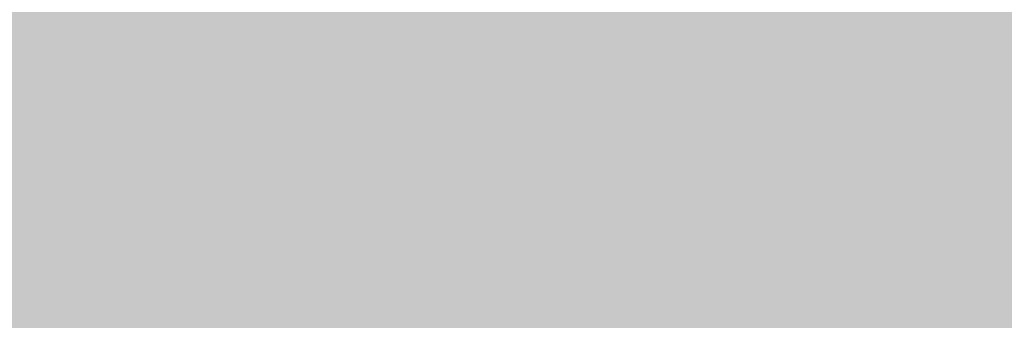
# Model space of a CAD drawing. Units: feet. Extents: x 3168 to 4724, y 827 to 1477.
# Tile 92 of 256: x 3275.224 to 3277.376, y 1098.344 to 1099.001. Entities that reach past the tile are written whole.
import ezdxf

# ---------------------------------------------------------------- set-up
doc = ezdxf.new("R2010")
doc.units = ezdxf.units.FT
doc.layers.add('A-ELEV', color=7, linetype='Continuous', lineweight=35)
doc.layers.add('A-ELEV-PATT', color=8, linetype='Continuous', lineweight=13)

msp = doc.modelspace()

# ---------------------------------------------------------------- hatches: boundary and pattern name
at = {"layer": 'A-ELEV-PATT'}
h = msp.add_hatch(color=256, dxfattribs=at)
h.dxf.hatch_style = 1
edge = h.paths.add_edge_path()
edge.add_ellipse((3552.9058, 979.2201), major_axis=(36.7449, 0), ratio=0.4848485, start_angle=0, end_angle=360)
edge = h.paths.add_edge_path()
edge.add_ellipse((3559.8916, 929.2523), major_axis=(36.7449, 0), ratio=0.4848485, start_angle=0, end_angle=360)
edge = h.paths.add_edge_path()
edge.add_line((3299.3168, 1198.6061), (3479.9167, 1198.6061))
edge.add_line((3479.9167, 1198.6061), (3479.9167, 1209.8686))
edge.add_spline(control_points=[(3479.9167, 1209.8686), (3464.3012, 1209.8686), (3448.6856, 1209.8686), (3410.9491, 1209.8686), (3388.8282, 1209.8686), (3355.6469, 1209.8686), (3344.5864, 1209.8686), (3327.9957, 1209.8686), (3322.4655, 1209.8686), (3314.1702, 1209.8686), (3311.4051, 1209.8686), (3307.2574, 1209.8686), (3305.8748, 1209.8686), (3303.801, 1209.8686), (3303.1097, 1209.8686), (3302.0728, 1209.8686), (3301.7272, 1209.8686), (3301.2087, 1209.8686), (3301.0359, 1209.8686), (3300.7767, 1209.8686), (3300.6903, 1209.8686), (3300.5606, 1209.8686), (3300.5174, 1209.8686), (3300.4526, 1209.8686), (3300.431, 1209.8686), (3300.3986, 1209.8686), (3300.3878, 1209.8686), (3300.3662, 1209.8686), (3300.3457, 1209.8686), (3300.3455, 1209.8686), (3300.3455, 1209.8686), (3300.3433, 1209.8686), (3300.3411, 1209.8686), (3300.3379, 1209.8686), (3300.3368, 1209.8686), (3300.3339, 1209.8686), (3300.3321, 1209.8686), (3300.3255, 1209.8686), (3300.3207, 1209.8686), (3300.3109, 1209.8686), (3300.306, 1209.8686), (3300.2905, 1209.8686), (3300.28, 1209.8686), (3300.2324, 1209.8688), (3300.1953, 1209.869), (3299.9511, 1209.8706), (3299.7448, 1209.8743), (3299.4368, 1209.8833), (3299.3344, 1209.8868), (3299.1811, 1209.8929), (3299.13, 1209.8951), (3298.6522, 1209.9168), (3298.2295, 1209.9457), (3297.6016, 1210.0024), (3297.3934, 1210.0235), (3297.0827, 1210.0583), (3296.9793, 1210.0705), (3296.293, 1210.1549), (3295.7181, 1210.2434), (3294.8687, 1210.3989), (3294.5877, 1210.4545), (3294.1693, 1210.5433), (3294.0304, 1210.5739), (3291.7071, 1211.1012), (3289.6536, 1211.8134), (3285.7763, 1213.564), (3283.9514, 1214.6035), (3280.5122, 1216.9801), (3278.8972, 1218.3176), (3276.3799, 1220.8295), (3275.416, 1221.9177), (3274.0393, 1223.7077), (3273.581, 1224.3495), (3273.1432, 1225.0163)], knot_values=[39.119033, 39.119033, 39.119033, 39.119033, 39.286353, 39.286353, 39.523379, 39.523379, 39.641892, 39.641892, 39.701148, 39.701148, 39.730777, 39.730777, 39.745591, 39.745591, 39.752998, 39.752998, 39.756701, 39.756701, 39.758553, 39.758553, 39.759479, 39.759479, 39.759942, 39.759942, 39.760173, 39.760173, 39.760289, 39.760289, 39.760405, 39.760405, 39.760463, 39.760463, 39.763389, 39.763389, 39.764851, 39.764851, 39.767304, 39.767304, 39.773825, 39.773825, 39.78057, 39.78057, 39.79477, 39.79477, 39.845194, 39.845194, 40.126715, 40.126715, 40.267476, 40.267476, 40.337856, 40.337856, 40.927023, 40.927023, 41.221606, 41.221606, 41.368898, 41.368898, 42.202622, 42.202622, 42.619485, 42.619485, 42.827916, 42.827916, 46.118323, 46.118323, 49.408731, 49.408731, 52.699139, 52.699139, 54.927489, 54.927489, 56.104228, 56.104228, 56.104228, 56.104228], weights=[1, 1, 1, 1, 1, 1, 1, 1, 1, 1, 1, 1, 1, 1, 1, 1, 1, 1, 1, 1, 1, 1, 1, 1, 1, 1, 1, 1, 1, 1, 1, 1, 1, 1, 1, 1, 1, 1, 1, 1, 1, 1, 1, 1, 1, 1, 1, 1, 1, 1, 1, 1, 1, 1, 1, 1, 1, 1, 1, 1, 1, 1, 1, 1, 1, 1, 1, 1, 1, 1, 1, 1, 1, 1], degree=3, periodic=0)
edge.add_line((3273.1432, 1225.0163), (3273.1432, 1099.0163))
edge.add_line((3273.1432, 1099.0163), (3299.3168, 1099.0163))
edge.add_line((3299.3168, 1099.0163), (3299.3168, 1198.6061))
edge = h.paths.add_edge_path()
edge.add_line((3304.7584, 1324.1581), (3479.9167, 1324.1581))
edge.add_line((3479.9167, 1324.1581), (3479.9167, 1335.7146))
edge.add_line((3479.9167, 1335.7146), (3269.1616, 1335.7146))
edge.add_spline(control_points=[(3269.1616, 1335.7146), (3264.0242, 1335.7146), (3258.3641, 1328.9582), (3259.2643, 1323.9003)], knot_values=[0, 0, 0, 0, 15.412191, 15.412191, 15.412191, 15.412191], degree=3, periodic=0)
edge.add_line((3259.2643, 1323.9003), (3265.5168, 1288.7691))
edge.add_line((3265.5168, 1288.7691), (3275.2651, 1261.5456))
edge.add_line((3275.2651, 1261.5456), (3304.7584, 1261.5456))
edge.add_line((3304.7584, 1261.5456), (3304.7584, 1324.1581))
h = msp.add_hatch(color=256, dxfattribs=at)
h.dxf.hatch_style = 1
h.paths.add_polyline_path([(3384.5252, 1099.0163), (3335.0292, 1099.0163), (3299.3168, 1099.0163), (3273.1432, 1099.0163), (3217.5654, 1099.0163), (3168.0693, 827.1163), (3335.0292, 827.1163)])

# ---------------------------------------------------------------- linework, layer by layer
at = {"layer": 'A-ELEV'}
msp.add_open_spline([(3808.5202, 1099.0163), (3808.5202, 1141.4132), (3808.5202, 1183.8102), (3808.5202, 1226.6353), (3808.5202, 1227.0636), (3808.5202, 1227.4918), (3811.4919, 1248.9947), (3814.4635, 1270.4975), (3817.4652, 1292.2176), (3817.4952, 1292.4348), (3817.5253, 1292.652), (3817.5728, 1310.1067), (3817.6203, 1327.5615), (3817.6679, 1345.0163), (3817.6679, 1345.458), (3817.6679, 1345.8996), (3817.6679, 1346.456), (3817.6679, 1346.5708), (3817.6679, 1346.7529), (3817.6679, 1346.8201), (3817.6679, 1346.9349), (3817.6679, 1346.9823), (3817.6679, 1347.0386), (3817.6679, 1347.0474), (3817.6679, 1347.0737), (3817.6679, 1347.0593), (3817.6679, 1347.0615), (3817.6679, 1347.0627), (3817.6679, 1347.066), (3817.6679, 1347.0683), (3817.6679, 1347.075), (3817.6679, 1347.0795), (3817.6678, 1347.0929), (3817.6678, 1347.1019), (3817.6678, 1347.1288), (3817.6677, 1347.1467), (3817.6674, 1347.2004), (3817.6672, 1347.2362), (3817.6661, 1347.3434), (3817.665, 1347.4147), (3817.6608, 1347.6281), (3817.6566, 1347.7697), (3817.64, 1348.1925), (3817.6235, 1348.4716), (3817.5591, 1349.3001), (3817.4961, 1349.8406), (3817.2554, 1351.4242), (3817.0263, 1352.4288), (3816.3069, 1354.8889), (3815.7437, 1356.2687), (3814.464, 1358.8192), (3813.7464, 1359.991), (3812.1958, 1362.1723), (3811.3622, 1363.1821), (3809.5888, 1365.069), (3808.6488, 1365.9461), (3806.6543, 1367.5796), (3805.5997, 1368.3362), (3803.3529, 1369.7223), (3802.1605, 1370.3524), (3799.6008, 1371.4536), (3798.2327, 1371.9255), (3795.2801, 1372.6346), (3793.6931, 1372.8721), (3791.8694, 1372.9265), (3791.7409, 1372.9292), (3791.3534, 1372.9341), (3791.0927, 1372.9329), (3790.3041, 1372.9151), (3789.7695, 1372.8842), (3789.2092, 1372.8302), (3789.1906, 1372.8284), (3789.1349, 1372.8229), (3789.0977, 1372.8191), (3789.0484, 1372.814), (3789.0364, 1372.8127), (3789.0003, 1372.8089), (3788.9761, 1372.8063), (3788.9494, 1372.8034), (3788.9468, 1372.8031), (3788.9426, 1372.8027), (3788.941, 1372.8025), (3788.9386, 1372.8022), (3788.9378, 1372.8021), (3788.9354, 1372.8019), (3788.8675, 1372.7944), (3788.7569, 1372.7822), (3788.7015, 1372.7761), (3788.5355, 1372.7579), (3788.4249, 1372.7457), (3788.0929, 1372.7092), (3787.8715, 1372.6848), (3787.2075, 1372.6118), (3786.7648, 1372.5631), (3785.4368, 1372.417), (3784.5515, 1372.3196), (3781.8954, 1372.0274), (3780.1247, 1371.8327), (3774.8126, 1371.2483), (3771.2713, 1370.8587), (3760.6471, 1369.69), (3753.5643, 1368.9109), (3732.316, 1366.5735), (3718.1504, 1365.0152), (3694.0068, 1362.3593), (3684.0287, 1361.2617), (3674.0506, 1360.1641), (3664.6007, 1360.1641), (3655.1508, 1360.1641), (3626.8011, 1360.1641), (3607.9013, 1360.1641), (3551.2019, 1360.1641), (3513.4023, 1360.1641), (3467.7252, 1360.1641), (3459.8476, 1360.1641), (3436.2149, 1360.1641), (3420.4597, 1360.1641), (3373.1943, 1360.1641), (3341.6839, 1360.1641), (3302.8482, 1360.1641), (3295.5227, 1360.1641), (3286.0383, 1360.1641), (3283.8794, 1360.1641), (3277.4026, 1360.1641), (3273.0848, 1360.1641), (3267.7329, 1360.1641), (3266.6988, 1360.1641), (3263.5965, 1360.1641), (3261.5284, 1360.1641), (3259.2369, 1360.1641), (3259.0137, 1360.1641), (3258.344, 1360.1641), (3257.8975, 1360.1641), (3257.431, 1360.1641), (3257.411, 1360.1641), (3257.3706, 1360.1641), (3257.3755, 1360.1641), (3257.3746, 1360.1641), (3257.3739, 1360.1641), (3257.372, 1360.1641), (3257.3706, 1360.1641), (3257.3667, 1360.1641), (3257.364, 1360.1641), (3257.3561, 1360.1641), (3257.3508, 1360.164), (3257.335, 1360.164), (3257.3244, 1360.164), (3257.2928, 1360.1639), (3257.2717, 1360.1638), (3257.2084, 1360.1634), (3257.1663, 1360.163), (3257.0402, 1360.1614), (3256.9563, 1360.1598), (3256.7055, 1360.1534), (3256.5392, 1360.147), (3256.0436, 1360.1219), (3255.7173, 1360.0971), (3254.7524, 1360.0005), (3254.128, 1359.9065), (3252.1801, 1359.5253), (3250.9416, 1359.144), (3248.6702, 1358.2433), (3247.6357, 1357.7238), (3245.7326, 1356.6035), (3244.8634, 1356.0021), (3243.2531, 1354.7429), (3242.512, 1354.0847), (3240.7511, 1352.3448), (3239.801, 1351.2296), (3238.0878, 1348.8724), (3237.3247, 1347.6304), (3235.9825, 1344.9716), (3235.4022, 1343.5549), (3234.5911, 1340.8155), (3234.3109, 1339.5435), (3233.9765, 1336.8026), (3233.9221, 1335.3309), (3234.1489, 1332.5913), (3234.3495, 1331.3672), (3234.7199, 1329.9994), (3234.7524, 1329.8834), (3234.8536, 1329.5348), (3234.9259, 1329.3017), (3235.0248, 1329.0026), (3235.0469, 1328.9369), (3235.0776, 1328.8472), (3235.0859, 1328.8232), (3235.1109, 1328.7511), (3235.1278, 1328.703), (3235.148, 1328.6462), (3235.1511, 1328.6376), (3235.1561, 1328.6235), (3235.1581, 1328.618), (3235.1602, 1328.612), (3235.1656, 1328.5969), (3235.1801, 1328.5565), (3235.1903, 1328.5281), (3235.2208, 1328.4429), (3235.2411, 1328.3862), (3235.3021, 1328.2159), (3235.3427, 1328.1023), (3235.4647, 1327.7617), (3235.546, 1327.5346), (3235.79, 1326.8534), (3235.9526, 1326.3992), (3236.4405, 1325.0367), (3236.7657, 1324.1284), (3237.7415, 1321.4034), (3238.392, 1319.5868), (3240.3435, 1314.1369), (3241.6445, 1310.5036), (3245.5476, 1299.6037), (3248.1496, 1292.3371), (3255.9557, 1270.5374), (3261.1598, 1256.0042), (3267.3876, 1238.612), (3268.4114, 1235.7529), (3269.5104, 1232.6839), (3269.5856, 1232.4739), (3269.7066, 1232.1359), (3269.7524, 1232.0079), (3269.8273, 1231.7987), (3269.8564, 1231.7176), (3269.9063, 1231.5781), (3269.9272, 1231.5198), (3269.9725, 1231.3934), (3269.9968, 1231.3254), (3270.0265, 1231.2425), (3270.0318, 1231.2277), (3270.0403, 1231.204), (3270.0392, 1231.207), (3270.0394, 1231.2066), (3270.0394, 1231.2064), (3270.0396, 1231.2058), (3270.0398, 1231.2055), (3270.0402, 1231.2043), (3270.0404, 1231.2036), (3270.0413, 1231.2013), (3270.0418, 1231.1998), (3270.0434, 1231.1953), (3270.0445, 1231.1922), (3270.0478, 1231.1832), (3270.0499, 1231.1771), (3270.0564, 1231.159), (3270.0608, 1231.147), (3270.0739, 1231.1108), (3270.0826, 1231.0867), (3270.1089, 1231.0144), (3270.1266, 1230.9663), (3270.1799, 1230.8225), (3270.2159, 1230.7269), (3270.3253, 1230.4415), (3270.4, 1230.2528), (3270.6292, 1229.6914), (3270.7889, 1229.3235), (3271.2865, 1228.2383), (3271.6431, 1227.5398), (3272.7759, 1225.5153), (3273.6142, 1224.2605), (3275.416, 1221.9177), (3276.3799, 1220.8295), (3278.8972, 1218.3176), (3280.5122, 1216.9801), (3283.9514, 1214.6035), (3285.7763, 1213.564), (3289.6536, 1211.8134), (3291.7071, 1211.1012), (3294.0304, 1210.5739), (3294.1693, 1210.5433), (3294.5877, 1210.4545), (3294.8687, 1210.3989), (3295.7181, 1210.2434), (3296.293, 1210.1549), (3296.9793, 1210.0705), (3297.0827, 1210.0583), (3297.3934, 1210.0235), (3297.6016, 1210.0024), (3298.2295, 1209.9457), (3298.6522, 1209.9168), (3299.13, 1209.8951), (3299.1811, 1209.8929), (3299.3344, 1209.8868), (3299.4368, 1209.8833), (3299.7448, 1209.8743), (3299.9511, 1209.8706), (3300.1953, 1209.869), (3300.2324, 1209.8688), (3300.28, 1209.8686), (3300.2905, 1209.8686), (3300.306, 1209.8686), (3300.3109, 1209.8686), (3300.3207, 1209.8686), (3300.3255, 1209.8686), (3300.3321, 1209.8686), (3300.3339, 1209.8686), (3300.3368, 1209.8686), (3300.3379, 1209.8686), (3300.3411, 1209.8686), (3300.3433, 1209.8686), (3300.3455, 1209.8686), (3300.3455, 1209.8686), (3300.3457, 1209.8686), (3300.3662, 1209.8686), (3300.3878, 1209.8686), (3300.3986, 1209.8686), (3300.431, 1209.8686), (3300.4526, 1209.8686), (3300.5174, 1209.8686), (3300.5606, 1209.8686), (3300.6903, 1209.8686), (3300.7767, 1209.8686), (3301.0359, 1209.8686), (3301.2087, 1209.8686), (3301.7272, 1209.8686), (3302.0728, 1209.8686), (3303.1097, 1209.8686), (3303.801, 1209.8686), (3305.8748, 1209.8686), (3307.2574, 1209.8686), (3311.4051, 1209.8686), (3314.1702, 1209.8686), (3322.4655, 1209.8686), (3327.9957, 1209.8686), (3344.5864, 1209.8686), (3355.6469, 1209.8686), (3388.8282, 1209.8686), (3410.9491, 1209.8686), (3477.3119, 1209.8686), (3521.5537, 1209.8686), (3566.8362, 1209.8686), (3567.8769, 1209.8686), (3570.999, 1209.8686), (3573.0804, 1209.8686), (3575.7814, 1209.8686), (3576.4009, 1209.8686), (3577.2958, 1209.8686), (3577.5712, 1209.8686), (3578.3971, 1209.8686), (3578.9478, 1209.8686), (3579.7565, 1209.8686), (3580.0145, 1209.8686), (3580.3427, 1209.8686), (3580.3269, 1209.8686), (3580.3272, 1209.8686), (3580.3273, 1209.8686), (3580.3278, 1209.8686), (3580.3281, 1209.8686), (3580.329, 1209.8686), (3580.3296, 1209.8686), (3580.3314, 1209.8686), (3580.3327, 1209.8686), (3580.3363, 1209.8686), (3580.3388, 1209.8686), (3580.3461, 1209.8686), (3580.351, 1209.8686), (3580.3657, 1209.8685), (3580.3754, 1209.8685), (3580.4048, 1209.8684), (3580.4244, 1209.8684), (3580.4832, 1209.8681), (3580.5224, 1209.8678), (3580.6404, 1209.8666), (3580.7192, 1209.8655), (3580.9563, 1209.8608), (3581.1152, 1209.8561), (3581.5942, 1209.8372), (3581.9164, 1209.8183), (3582.8899, 1209.7424), (3583.548, 1209.6662), (3585.5318, 1209.3606), (3586.8672, 1209.0539), (3589.4715, 1208.2525), (3590.7402, 1207.7579), (3591.9955, 1207.1588), (3592.0578, 1207.1287), (3592.2442, 1207.038), (3592.3677, 1206.9766), (3592.7353, 1206.7904), (3592.9768, 1206.6631), (3593.2445, 1206.5164), (3593.2747, 1206.4998), (3593.3651, 1206.4498), (3593.4251, 1206.4163), (3593.6043, 1206.3153), (3593.7227, 1206.2472), (3593.8572, 1206.1684), (3593.8744, 1206.1583), (3593.9257, 1206.128), (3593.9599, 1206.1078), (3594.0621, 1206.0469), (3594.1298, 1206.0061), (3594.2084, 1205.9582), (3594.2197, 1205.9513), (3594.2534, 1205.9307), (3594.2758, 1205.9169), (3594.343, 1205.8755), (3594.3876, 1205.8479), (3594.4336, 1205.819), (3594.4353, 1205.818), (3594.4402, 1205.8149), (3594.4435, 1205.8129), (3594.4471, 1205.8106), (3594.4475, 1205.8103), (3594.4487, 1205.8096), (3594.4495, 1205.8091), (3594.4504, 1205.8086), (3594.4505, 1205.8085), (3594.4506, 1205.8084), (3594.4674, 1205.7979), (3594.4933, 1205.7817), (3594.5062, 1205.7736), (3594.545, 1205.7492), (3594.5709, 1205.733), (3594.6485, 1205.6844), (3594.7002, 1205.652), (3594.8554, 1205.5547), (3594.9589, 1205.4898), (3595.2694, 1205.2953), (3595.4763, 1205.1656), (3596.0972, 1204.7765), (3596.5111, 1204.5171), (3597.7528, 1203.7388), (3598.5807, 1203.22), (3601.0642, 1201.6636), (3602.7198, 1200.6259), (3607.6868, 1197.513), (3610.9981, 1195.4377), (3620.932, 1189.2119), (3627.5546, 1185.0614), (3647.4225, 1172.6097), (3660.6678, 1164.3086), (3700.4035, 1139.4053), (3726.894, 1122.8031), (3757.2057, 1103.8061), (3761.027, 1101.4112), (3764.8482, 1099.0163), (3745.3283, 1099.0163), (3725.8083, 1099.0163), (3706.2884, 1099.0163), (3706.2884, 1108.4532), (3706.2884, 1117.8902), (3706.2884, 1127.3271), (3710.7508, 1127.3271), (3715.2131, 1127.3271), (3719.6755, 1127.3271)], degree=3, knots=[0, 0, 0, 0, 0.982037, 0.982037, 0.991957, 0.991957, 0.991957, 1.966522, 1.966522, 1.976367, 1.976367, 1.976367, 2.976367, 2.976367, 2.976367, 3.00169, 3.00169, 3.008272, 3.008272, 3.012129, 3.012129, 3.014851, 3.014851, 3.015353, 3.015353, 3.016359, 3.016359, 3.017365, 3.017365, 3.019376, 3.019376, 3.023398, 3.023398, 3.031442, 3.031442, 3.047531, 3.047531, 3.079708, 3.079708, 3.144063, 3.144063, 3.272772, 3.272772, 3.53019, 3.53019, 4.045026, 4.045026, 5.074698, 5.074698, 6.700878, 6.700878, 8.327058, 8.327058, 9.953238, 9.953238, 11.579418, 11.579418, 13.205598, 13.205598, 14.831778, 14.831778, 16.457958, 16.457958, 18.084138, 18.084138, 18.206872, 18.206872, 18.45234, 18.45234, 18.943275, 18.943275, 18.960093, 18.960093, 18.993729, 18.993729, 19.00461, 19.00461, 19.026374, 19.026374, 19.028737, 19.028737, 19.03018, 19.03018, 19.030897, 19.030897, 19.032332, 19.032332, 19.033766, 19.033766, 19.036636, 19.036636, 19.042374, 19.042374, 19.053851, 19.053851, 19.076805, 19.076805, 19.122714, 19.122714, 19.21453, 19.21453, 19.398163, 19.398163, 19.765429, 19.765429, 20.024128, 20.024128, 20.024128, 20.092031, 20.092031, 20.227836, 20.227836, 20.499446, 20.499446, 20.556051, 20.556051, 20.66926, 20.66926, 20.895678, 20.895678, 20.948316, 20.948316, 20.963829, 20.963829, 20.994855, 20.994855, 21.002285, 21.002285, 21.017146, 21.017146, 21.01875, 21.01875, 21.021959, 21.021959, 21.022102, 21.022102, 21.022249, 21.022249, 21.022708, 21.022708, 21.023627, 21.023627, 21.025464, 21.025464, 21.029138, 21.029138, 21.036486, 21.036486, 21.051183, 21.051183, 21.080575, 21.080575, 21.139361, 21.139361, 21.256932, 21.256932, 21.492073, 21.492073, 21.962356, 21.962356, 23.01002, 23.01002, 24.057684, 24.057684, 25.105348, 25.105348, 26.153011, 26.153011, 27.776787, 27.776787, 29.400562, 29.400562, 31.024337, 31.024337, 32.278801, 32.278801, 33.533265, 33.533265, 34.467568, 34.467568, 34.553971, 34.553971, 34.726776, 34.726776, 34.775309, 34.775309, 34.793079, 34.793079, 34.82862, 34.82862, 34.834979, 34.834979, 34.839039, 34.839039, 34.839411, 34.839411, 34.840285, 34.840285, 34.842034, 34.842034, 34.845531, 34.845531, 34.852525, 34.852525, 34.866512, 34.866512, 34.894488, 34.894488, 34.950439, 34.950439, 35.062342, 35.062342, 35.286147, 35.286147, 35.733758, 35.733758, 35.821815, 35.821815, 35.828283, 35.828283, 35.832225, 35.832225, 35.834724, 35.834724, 35.836521, 35.836521, 35.838617, 35.838617, 35.839073, 35.839073, 35.839345, 35.839345, 35.839617, 35.839617, 35.840161, 35.840161, 35.841249, 35.841249, 35.843425, 35.843425, 35.847778, 35.847778, 35.856482, 35.856482, 35.873891, 35.873891, 35.908709, 35.908709, 35.978345, 35.978345, 36.117617, 36.117617, 36.396161, 36.396161, 36.953248, 36.953248, 38.067423, 38.067423, 40.295772, 40.295772, 42.524122, 42.524122, 45.81453, 45.81453, 49.104937, 49.104937, 52.395345, 52.395345, 52.603776, 52.603776, 53.020639, 53.020639, 53.854363, 53.854363, 54.001655, 54.001655, 54.296238, 54.296238, 54.885405, 54.885405, 54.955785, 54.955785, 55.096546, 55.096546, 55.378067, 55.378067, 55.42849, 55.42849, 55.442691, 55.442691, 55.449436, 55.449436, 55.455957, 55.455957, 55.458409, 55.458409, 55.459872, 55.459872, 55.462798, 55.462798, 55.462856, 55.462856, 55.462972, 55.462972, 55.463088, 55.463088, 55.463319, 55.463319, 55.463782, 55.463782, 55.464708, 55.464708, 55.46656, 55.46656, 55.470263, 55.470263, 55.47767, 55.47767, 55.492484, 55.492484, 55.522112, 55.522112, 55.581369, 55.581369, 55.699882, 55.699882, 55.936907, 55.936907, 56.410959, 56.410959, 56.42211, 56.42211, 56.444413, 56.444413, 56.451051, 56.451051, 56.454001, 56.454001, 56.459901, 56.459901, 56.462666, 56.462666, 56.463418, 56.463418, 56.464171, 56.464171, 56.465675, 56.465675, 56.468684, 56.468684, 56.474702, 56.474702, 56.486738, 56.486738, 56.51081, 56.51081, 56.558955, 56.558955, 56.655243, 56.655243, 56.847821, 56.847821, 57.232975, 57.232975, 58.003284, 58.003284, 59.543901, 59.543901, 62.625137, 62.625137, 68.787607, 68.787607, 74.950078, 74.950078, 75.27336, 75.27336, 75.919923, 75.919923, 77.213051, 77.213051, 77.377769, 77.377769, 77.707206, 77.707206, 78.366079, 78.366079, 78.462532, 78.462532, 78.655436, 78.655436, 79.041245, 79.041245, 79.105735, 79.105735, 79.234714, 79.234714, 79.492672, 79.492672, 79.502197, 79.502197, 79.521249, 79.521249, 79.523534, 79.523534, 79.528103, 79.528103, 79.528682, 79.528682, 79.528885, 79.528885, 79.529089, 79.529089, 79.529495, 79.529495, 79.530308, 79.530308, 79.531935, 79.531935, 79.535187, 79.535187, 79.541693, 79.541693, 79.554704, 79.554704, 79.580725, 79.580725, 79.632769, 79.632769, 79.736856, 79.736856, 79.94503, 79.94503, 80.361377, 80.361377, 80.421435, 80.421435, 80.421435, 81.421435, 81.421435, 81.421435, 82.421435, 82.421435, 82.421435, 83.421435, 83.421435, 83.421435, 83.421435], dxfattribs=at)

doc.saveas('drawing.dxf')
